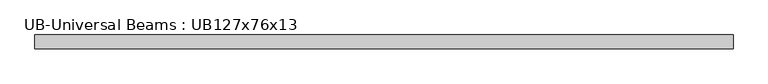
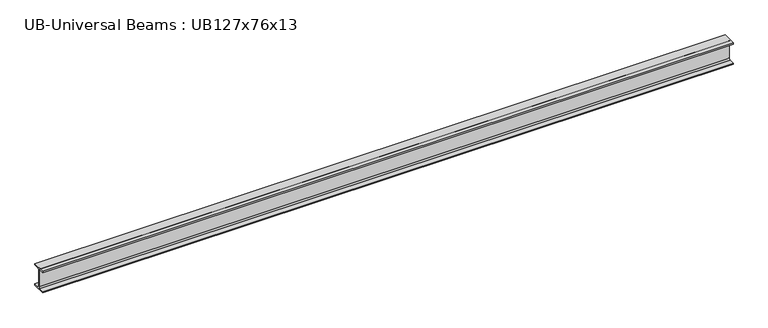
"""IFC4 building model written with IfcOpenShell, lengths in millimetres: member geometry, UB-Universal Beams : UB127x76x13."""

from ifc_helpers import new_model, si_unit, point, frame, frame_2d, origin, place, context, project, spatial, polyline, circle_curve, trimmed, segment, composite_curve, outline, extrude, source, transform, mapped, element, save


def ub_universal_beams_ub127x76x13_debcaab1(model_context):
    return source(origin(), model_context, "Body", "SweptSolid", [
        extrude(outline(composite_curve([segment(polyline([(-38.0, -55.9), (-9.6, -55.9)]), True, "CONTINUOUS"), segment(trimmed(circle_curve(frame_2d((-9.6, -48.3)), 7.6), [point((-9.6, -55.9))], [point((-2.0, -48.3))], True, "CARTESIAN"), True, "CONTINUOUS"), segment(polyline([(-2.0, -48.3), (-2.0, 48.3)]), True, "CONTINUOUS"), segment(trimmed(circle_curve(frame_2d((-9.6, 48.3)), 7.6), [point((-2.0, 48.3))], [point((-9.6, 55.9))], True, "CARTESIAN"), True, "CONTINUOUS"), segment(polyline([(-9.6, 55.9), (-38.0, 55.9), (-38.0, 63.5), (38.0, 63.5), (38.0, 55.9), (9.6, 55.9)]), True, "CONTINUOUS"), segment(trimmed(circle_curve(frame_2d((9.6, 48.3)), 7.6), [point((9.6, 55.9))], [point((2.0, 48.3))], True, "CARTESIAN"), True, "CONTINUOUS"), segment(polyline([(2.0, 48.3), (2.0, -48.3)]), True, "CONTINUOUS"), segment(trimmed(circle_curve(frame_2d((9.6, -48.3)), 7.6), [point((2.0, -48.3))], [point((9.6, -55.9))], True, "CARTESIAN"), True, "CONTINUOUS"), segment(polyline([(9.6, -55.9), (38.0, -55.9), (38.0, -63.5), (-38.0, -63.5), (-38.0, -55.9)]), True, "CONTINUOUS")], self_intersect=False)), frame((-1922.65, 0.0, 0.0), z_axis=(1.0, 0.0, 0.0), x_axis=(0.0, 1.0, 0.0)), (0.0, 0.0, 1.0), 3845.3),
    ])


if __name__ == "__main__":
    model = new_model("IFC4")
    model_context = context("Model", 3, world=origin())
    ifc_project = project(units=[si_unit("LENGTHUNIT", "METRE", prefix="MILLI")], contexts=[model_context])
    site = spatial("IfcSite", under=ifc_project)
    building = spatial("IfcBuilding", under=site)
    placement = place(None, origin())
    ub_universal_beams_ub127x76x13_shape = ub_universal_beams_ub127x76x13_debcaab1(model_context)
    element("IfcMember", 1, ObjectType="UB-Universal Beams : UB127x76x13", at=placement, inside=building, context=model_context, shape_type="MappedRepresentation", body=[
        mapped(ub_universal_beams_ub127x76x13_shape, transform((0.0, 0.0, 0.0), x_axis=(1.0, 0.0, 0.0), y_axis=(0.0, 1.0, 0.0), z_axis=(0.0, 0.0, 1.0))),
    ])
    save(model, "model.ifc")

# Revit data of these elements
# Type "UB-Universal Beams : UB127x76x13"
#   Section Name Key = "UB127X76X13"
#   Width = 7.6 cm
#   Web Thickness = 0.4 cm
#   Web Fillet = 0.76 cm
#   Warping Constant = 2000.0 cm⁶
#   Torsional Moment of Inertia = 2.85 cm⁴
#   Section Area = 16.5 cm²
#   Plastic Modulus weak axis = 22.6 cm³
#   Plastic Modulus strong axis = 84.2 cm³
#   Nominal Weight = 13.00 kgf/m
#   Moment of Inertia weak axis = 55.70 cm⁴
#   Moment of Inertia strong axis = 473.00 cm⁴
#   Height = 12.7 cm
#   Flange Thickness = 0.76 cm
#   Elastic Modulus weak axis = 14.7 cm³
#   Elastic Modulus strong axis = 74.6 cm³
#   Centroid Vertical = 6.35 cm
#   Centroid Horizontal = 3.8 cm
#   Bolt Spacing = 4.0 cm
#   Length [instance default] = 1.5 m
#   Structural Material [instance default] = Metal - Steel 43-275
#   Type Comments = ""
#   Assembly Code = ""
# Element 1 (IfcMember, "UB-Universal Beams : UB127x76x13")
#   Materials on its faces: "Metal - Steel 43-275"
# Materials
#   "Metal - Steel 43-275": class "Metal", colour RGB 247 247 247, transparency 0, Cost = 0
